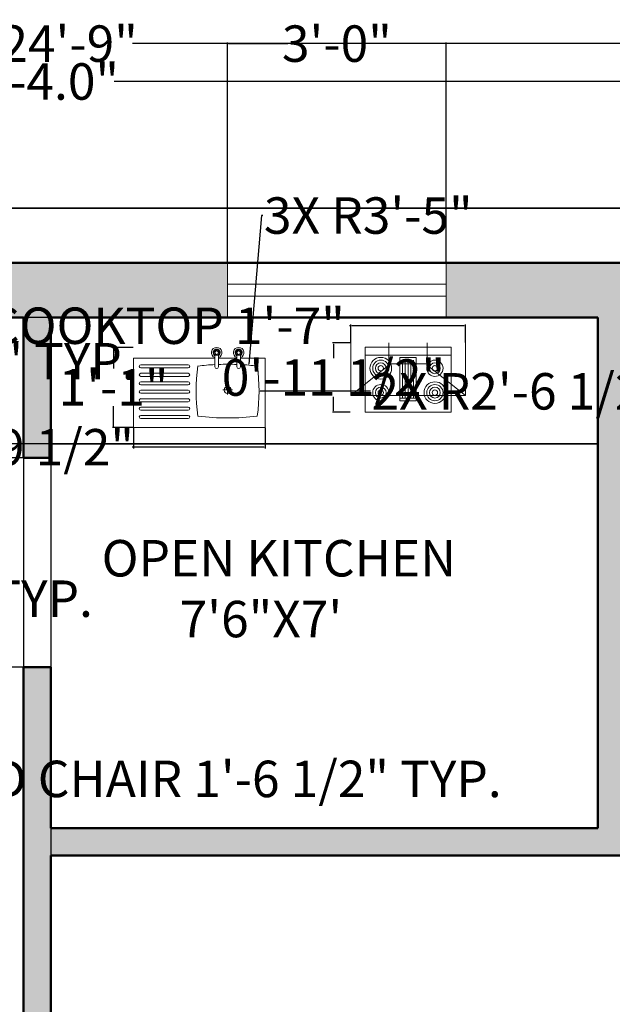
# Model space of a CAD drawing. Units: inches. Extents: x 3398 to 3816, y 15195 to 15771.
# Tile 9 of 10: x 3606 to 3703, y 15609 to 15771. Entities that reach past the tile are written whole.
import ezdxf

# ---------------------------------------------------------------- set-up
doc = ezdxf.new("R2010")
doc.units = ezdxf.units.IN
doc.header["$MEASUREMENT"] = 0
for name, color, linetype, lineweight in [('A-ANNO-DIMS', 2, 'Continuous', 18), ('A-AREA-IDEN', 7, 'Continuous', 25), ('A-EQPM', 8, 'Continuous', 18), ('A-FLOR-CASE', 7, 'Continuous', 25), ('A-FLOR-FIXT', 8, 'Continuous', 18), ('A-GLAZ', 4, 'Continuous', 18), ('A-WALL', 7, 'Continuous', 50), ('A-WALL-PATT', 252, 'Continuous', 13), ('C-PROP', 7, 'Continuous', 35)]:
    doc.layers.add(name, color=color, linetype=linetype, lineweight=lineweight)
doc.styles.get("Standard").update_dxf_attribs({"font": 'arial.ttf'})
doc.dimstyles.get("Standard").update_dxf_attribs({"dimtxt": 6, "dimasz": 0.18, "dimexe": 0.18, "dimexo": 0.0625, "dimgap": 0.09, "dimtad": 0, "dimtih": 1, "dimtoh": 1, "dimdec": 1, "dimzin": 0, "dimdsep": 46, "dimlunit": 3, "dimtxsty": 'Standard', "dimcen": 0.09, "dimadec": 0, "dimazin": 0, "dimtfac": 1, "dimtdec": 1, "dimtofl": 0, "dimtmove": 0, "dimatfit": 3, "dimfxl": 1, "dimtolj": 1, "dimtzin": 0, "dimarcsym": 0})

# ---------------------------------------------------------------- blocks, each defined once
blk = doc.blocks.new('chimmne')
for p, q in [((17.89, 6.07), (-18.11, 6.07)), ((-18.11, 6.07), (-18.11, -10.43)), ((-6.16, -3.43), (-18.11, 6.07)), ((5.94, -3.43), (17.89, 6.07)), ((17.89, 6.07), (17.89, -10.43)), ((-6.16, -3.43), (-6.16, -10.43)), ((5.94, -3.82), (-6.16, -3.82)), ((5.94, -3.43), (5.94, -10.43))]:
    blk.add_line(p, q)
for points in [[(-13.61, -9.12), (-13.61, 11.28), (13.39, 11.28), (13.39, -9.12)], [(-2.66, -5.87), (-2.66, 7.73), (2.44, 7.73), (2.44, -5.87)]]:
    blk.add_lwpolyline(points, close=True)
for points in [[(-2.66, 6.88), (2.44, 6.88)], [(-1.81, 6.88), (-1.81, -5.02)], [(-0.96, -5.02), (-0.96, 6.88)], [(-0.11, 6.88), (-0.11, -5.02)], [(0.74, -5.02), (0.74, 6.88)], [(1.59, 6.88), (1.59, -5.02)], [(13.39, -6.57), (-13.61, -6.57)]]:
    blk.add_lwpolyline(points)
for centre, radius in [((-8.55, 5.18), 3.4), ((-8.55, 5.18), 2.55), ((-8.55, 5.18), 1.7), ((8.44, 5.18), 2.55), ((8.44, 5.18), 1.7), ((-8.55, 5.18), 0.85), ((8.44, 5.18), 0.85), ((-8.55, -2.47), 2.55), ((8.44, -2.47), 3.4), ((8.44, -2.47), 2.55), ((-8.55, -2.47), 1.7), ((-8.55, -2.47), 0.85), ((8.44, -2.47), 1.7), ((8.44, -2.47), 0.85)]:
    blk.add_circle(centre, radius)
blk = doc.blocks.new('A$C799204C7')
for p, q in [((0, 34.2), (17.99, 34.2)), ((0, 0), (0, 34.2)), ((17.99, 13.08), (17.99, 34.2)), ((2.32, 20.01), (2.32, 32.27)), ((3.13, 20.01), (3.13, 32.27)), ((4.48, 20.01), (4.48, 32.27)), ((5.29, 20.01), (5.29, 32.27)), ((6.64, 20.01), (6.64, 32.27)), ((7.45, 20.01), (7.45, 32.27)), ((8.85, 20.01), (8.85, 32.27)), ((9.66, 20.01), (9.66, 32.27)), ((11.01, 20.01), (11.01, 32.27)), ((11.82, 20.01), (11.82, 32.27)), ((13.22, 20.01), (13.22, 32.27)), ((14.03, 20.01), (14.03, 32.27)), ((15.42, 20.01), (15.42, 32.27)), ((16.24, 20.01), (16.24, 32.27)), ((18.59, 13.08), (15.71, 13.08)), ((9.73, 11), (9.73, 8.54)), ((15.71, 12.17), (18.59, 12.17)), ((17.99, 7.36), (17.99, 12.17)), ((8.52, 9.77), (10.9, 9.77)), ((18.59, 7.36), (15.71, 7.36)), ((15.71, 6.45), (18.59, 6.45)), ((17.99, 0), (17.99, 6.45)), ((0, 0), (17.99, 0))]:
    blk.add_line(p, q)
for centre, radius in [((19.38, 12.62), 0.684), ((19.38, 12.62), 0.456), ((9.7, 9.77), 0.916), ((19.38, 6.91), 0.684), ((19.38, 6.91), 0.456)]:
    blk.add_circle(centre, radius)
for centre, radius, start, end in [((2.72, 32.27), 0.407, 0, 180), ((4.88, 32.27), 0.407, 0, 180), ((7.05, 32.27), 0.407, 0, 180), ((9.25, 32.27), 0.407, 0, 180), ((11.42, 32.27), 0.407, 0, 180), ((13.62, 32.27), 0.407, 0, 180), ((15.83, 32.27), 0.407, 0, 180), ((2.72, 20.01), 0.407, 180, 0), ((9.53, -30.19), 48.1, 82.3437, 97.8966), ((4.88, 20.01), 0.407, 180, 0), ((7.05, 20.01), 0.407, 180, 0), ((9.25, 20.01), 0.407, 180, 0), ((11.42, 20.01), 0.407, 180, 0), ((13.62, 20.01), 0.407, 180, 0), ((15.83, 20.01), 0.407, 180, 0), ((67.33, 9.77), 64.88, 173.1952, 186.8048), ((-48.51, 9.77), 64.88, 2.9208, 6.8048), ((15.71, 12.62), 0.456, 90, 270), ((19.38, 12.62), 1.37, 199.6514, 160.3603), ((19.38, 12.62), 0.911, 210.3431, 149.7554), ((-48.51, 9.77), 64.88, 357.8723, 2.115), ((19.38, 6.91), 1.37, 199.6514, 160.3603), ((19.38, 6.91), 0.911, 210.3431, 149.7554), ((15.71, 6.91), 0.456, 90, 270), ((-48.51, 9.77), 64.88, 353.1952, 357.0665), ((9.53, 49.73), 48.1, 262.1034, 277.6563)]:
    blk.add_arc(centre, radius, start, end)
blk = doc.blocks.new('*D4')
at = {"layer": 'A-ANNO-DIMS', "color": 0, "lineweight": -2, "transparency": 16777216}
for p, q in [((3443.19, 15739.58), (3443.19, 15760.52)), ((3771.19, 15739.58), (3771.19, 15760.52)), ((3443.37, 15760.34), (3593.25, 15760.34)), ((3771.01, 15760.34), (3621.13, 15760.34))]:
    blk.add_line(p, q, dxfattribs=at)
at = {"layer": 'A-ANNO-DIMS', "color": 0, "transparency": 16777216}
for points in [[(3443.37, 15760.37), (3443.37, 15760.31), (3443.19, 15760.34)], [(3771.01, 15760.37), (3771.01, 15760.31), (3771.19, 15760.34)]]:
    blk.add_solid(points, dxfattribs=at)
at = {"layer": 'Defpoints', "color": 0, "transparency": 16777216}
for p in [(3771.19, 15760.34), (3443.19, 15739.52), (3771.19, 15739.52)]:
    blk.add_point(p, dxfattribs=at)
at = {"layer": 'A-ANNO-DIMS', "color": 0, "transparency": 16777216, "insert": (3607.19, 15760.34), "char_height": 6, "attachment_point": 5}
blk.add_mtext('\\A1;27\'-4.0"', dxfattribs=at)
blk = doc.blocks.new('*D14')
at = {"layer": 'A-ANNO-DIMS', "color": 0, "lineweight": -2, "transparency": 16777216}
for p, q in [((3515.96, 15721.46), (3515.96, 15714.14)), ((3563.96, 15721.46), (3563.96, 15714.14)), ((3516.14, 15714.32), (3563.78, 15714.32)), ((3563.96, 15714.32), (3564.14, 15714.32))]:
    blk.add_line(p, q, dxfattribs=at)
at = {"layer": 'A-ANNO-DIMS', "color": 0, "transparency": 16777216}
for points in [[(3516.14, 15714.35), (3516.14, 15714.29), (3515.96, 15714.32)], [(3563.78, 15714.35), (3563.78, 15714.29), (3563.96, 15714.32)]]:
    blk.add_solid(points, dxfattribs=at)
at = {"layer": 'Defpoints', "color": 0, "transparency": 16777216}
for p in [(3515.96, 15721.52), (3563.96, 15721.52), (3563.96, 15714.32)]:
    blk.add_point(p, dxfattribs=at)
at = {"layer": 'A-ANNO-DIMS', "color": 0, "transparency": 16777216, "insert": (3595.08, 15714.32), "char_height": 6, "attachment_point": 5}
blk.add_mtext('\\A1;SASH 4\'-0" TYP.', dxfattribs=at)
blk = doc.blocks.new('*D16')
at = {"layer": 'A-ANNO-DIMS', "color": 0, "lineweight": -2, "transparency": 16777216}
for p, q in [((3521.16, 15677.98), (3521.16, 15675.08)), ((3539.72, 15677.98), (3539.72, 15675.08)), ((3521.34, 15675.26), (3539.54, 15675.26)), ((3539.72, 15675.26), (3539.9, 15675.26))]:
    blk.add_line(p, q, dxfattribs=at)
at = {"layer": 'A-ANNO-DIMS', "color": 0, "transparency": 16777216}
for points in [[(3521.34, 15675.29), (3521.34, 15675.23), (3521.16, 15675.26)], [(3539.54, 15675.29), (3539.54, 15675.23), (3539.72, 15675.26)]]:
    blk.add_solid(points, dxfattribs=at)
at = {"layer": 'Defpoints', "color": 0, "transparency": 16777216}
for p in [(3521.16, 15678.04), (3539.72, 15678.04), (3539.72, 15675.26)]:
    blk.add_point(p, dxfattribs=at)
at = {"layer": 'A-ANNO-DIMS', "color": 0, "transparency": 16777216, "insert": (3579.44, 15675.26), "char_height": 6, "attachment_point": 5}
blk.add_mtext('\\A1;CHAIR 1\'-6 1/2" TYP.', dxfattribs=at)
blk = doc.blocks.new('*D18')
at = {"layer": 'A-ANNO-DIMS', "color": 0, "lineweight": -2, "transparency": 16777216}
for p, q in [((3548.56, 15642.88), (3548.56, 15645.79)), ((3548.74, 15645.61), (3566.94, 15645.61)), ((3567.12, 15642.88), (3567.12, 15645.79)), ((3567.12, 15645.61), (3567.3, 15645.61))]:
    blk.add_line(p, q, dxfattribs=at)
at = {"layer": 'A-ANNO-DIMS', "color": 0, "transparency": 16777216}
for points in [[(3548.74, 15645.64), (3548.74, 15645.58), (3548.56, 15645.61)], [(3566.94, 15645.64), (3566.94, 15645.58), (3567.12, 15645.61)]]:
    blk.add_solid(points, dxfattribs=at)
at = {"layer": 'Defpoints', "color": 0, "transparency": 16777216}
for p in [(3567.12, 15645.61), (3548.56, 15642.82), (3567.12, 15642.82)]:
    blk.add_point(p, dxfattribs=at)
at = {"layer": 'A-ANNO-DIMS', "color": 0, "transparency": 16777216, "insert": (3627.67, 15645.61), "char_height": 6, "attachment_point": 5}
blk.add_mtext('\\A1;TRIMMED CHAIR 1\'-6 1/2" TYP.', dxfattribs=at)
blk = doc.blocks.new('*D30')
at = {"layer": 'A-ANNO-DIMS', "color": 0, "lineweight": -2, "transparency": 16777216}
for p, q in [((3660.03, 15720.16), (3659.85, 15720.16)), ((3660.03, 15717.39), (3660.03, 15720.34)), ((3678.72, 15720.16), (3660.21, 15720.16)), ((3678.9, 15717.39), (3678.9, 15720.34))]:
    blk.add_line(p, q, dxfattribs=at)
at = {"layer": 'A-ANNO-DIMS', "color": 0, "transparency": 16777216}
for points in [[(3660.21, 15720.19), (3660.21, 15720.13), (3660.03, 15720.16)], [(3678.72, 15720.19), (3678.72, 15720.13), (3678.9, 15720.16)]]:
    blk.add_solid(points, dxfattribs=at)
at = {"layer": 'Defpoints', "color": 0, "transparency": 16777216}
for p in [(3660.03, 15720.16), (3660.03, 15717.33), (3678.9, 15717.33)]:
    blk.add_point(p, dxfattribs=at)
at = {"layer": 'A-ANNO-DIMS', "color": 0, "transparency": 16777216, "insert": (3629.7, 15720.16), "char_height": 6, "attachment_point": 5}
blk.add_mtext('\\A1;COOKTOP 1\'-7"', dxfattribs=at)
blk = doc.blocks.new('*D31')
at = {"layer": 'A-ANNO-DIMS', "color": 0, "lineweight": -2, "transparency": 16777216}
for p, q in [((3659.97, 15717.33), (3657.02, 15717.33)), ((3657.2, 15717.15), (3657.2, 15714.84)), ((3657.2, 15706.14), (3657.2, 15708.45)), ((3659.97, 15705.96), (3657.02, 15705.96))]:
    blk.add_line(p, q, dxfattribs=at)
at = {"layer": 'A-ANNO-DIMS', "color": 0, "transparency": 16777216}
for points in [[(3657.17, 15717.15), (3657.23, 15717.15), (3657.2, 15717.33)], [(3657.17, 15706.14), (3657.23, 15706.14), (3657.2, 15705.96)]]:
    blk.add_solid(points, dxfattribs=at)
at = {"layer": 'Defpoints', "color": 0, "transparency": 16777216}
for p in [(3660.03, 15717.33), (3657.2, 15705.96), (3660.03, 15705.96)]:
    blk.add_point(p, dxfattribs=at)
at = {"layer": 'A-ANNO-DIMS', "color": 0, "transparency": 16777216, "insert": (3657.2, 15711.64), "char_height": 6, "attachment_point": 5}
blk.add_mtext('\\A1;0\'-11 1/2"', dxfattribs=at)
blk = doc.blocks.new('*D32')
at = {"layer": 'A-ANNO-DIMS', "color": 0, "lineweight": -2, "transparency": 16777216}
for p, q in [((3624.27, 15703.37), (3624.27, 15699.99)), ((3645.98, 15703.37), (3645.98, 15699.99)), ((3624.27, 15700.17), (3624.09, 15700.17)), ((3645.8, 15700.17), (3624.45, 15700.17))]:
    blk.add_line(p, q, dxfattribs=at)
at = {"layer": 'A-ANNO-DIMS', "color": 0, "transparency": 16777216}
for points in [[(3624.45, 15700.2), (3624.45, 15700.14), (3624.27, 15700.17)], [(3645.8, 15700.2), (3645.8, 15700.14), (3645.98, 15700.17)]]:
    blk.add_solid(points, dxfattribs=at)
at = {"layer": 'Defpoints', "color": 0, "transparency": 16777216}
for p in [(3624.27, 15703.43), (3645.98, 15703.43), (3624.27, 15700.17)]:
    blk.add_point(p, dxfattribs=at)
at = {"layer": 'A-ANNO-DIMS', "color": 0, "transparency": 16777216, "insert": (3598.1, 15700.17), "char_height": 6, "attachment_point": 5}
blk.add_mtext('\\A1;SINK 1\'-9 1/2"', dxfattribs=at)
blk = doc.blocks.new('*D33')
at = {"layer": 'A-ANNO-DIMS', "color": 0, "lineweight": -2, "transparency": 16777216}
for p, q in [((3624.21, 15716.6), (3620.83, 15716.6)), ((3621.01, 15716.42), (3621.01, 15713.12)), ((3621.01, 15703.61), (3621.01, 15706.91)), ((3624.21, 15703.43), (3620.83, 15703.43))]:
    blk.add_line(p, q, dxfattribs=at)
at = {"layer": 'A-ANNO-DIMS', "color": 0, "transparency": 16777216}
for points in [[(3620.98, 15716.42), (3621.04, 15716.42), (3621.01, 15716.6)], [(3620.98, 15703.61), (3621.04, 15703.61), (3621.01, 15703.43)]]:
    blk.add_solid(points, dxfattribs=at)
at = {"layer": 'Defpoints', "color": 0, "transparency": 16777216}
for p in [(3621.01, 15716.6), (3624.27, 15716.6), (3624.27, 15703.43)]:
    blk.add_point(p, dxfattribs=at)
at = {"layer": 'A-ANNO-DIMS', "color": 0, "transparency": 16777216, "insert": (3621.01, 15710.02), "char_height": 6, "attachment_point": 5}
blk.add_mtext('\\A1;1\'-1"', dxfattribs=at)
blk = doc.blocks.new('*D36')
at = {"layer": 'A-ANNO-DIMS', "color": 0, "lineweight": -2, "transparency": 16777216}
for p, q in [((3465.19, 15730.58), (3465.19, 15766.75)), ((3465.37, 15766.57), (3603.24, 15766.57)), ((3762.01, 15766.57), (3624.14, 15766.57)), ((3762.19, 15730.58), (3762.19, 15766.75))]:
    blk.add_line(p, q, dxfattribs=at)
at = {"layer": 'A-ANNO-DIMS', "color": 0, "transparency": 16777216}
for points in [[(3465.37, 15766.6), (3465.37, 15766.54), (3465.19, 15766.57)], [(3762.01, 15766.6), (3762.01, 15766.54), (3762.19, 15766.57)]]:
    blk.add_solid(points, dxfattribs=at)
at = {"layer": 'Defpoints', "color": 0, "transparency": 16777216}
for p in [(3762.19, 15766.57), (3465.19, 15730.52), (3762.19, 15730.52)]:
    blk.add_point(p, dxfattribs=at)
at = {"layer": 'A-ANNO-DIMS', "color": 0, "transparency": 16777216, "insert": (3613.69, 15766.57), "char_height": 6, "attachment_point": 5}
blk.add_mtext('\\A1;24\'-9"', dxfattribs=at)
blk = doc.blocks.new('*D42')
at = {"layer": 'A-ANNO-DIMS', "color": 0, "lineweight": -2, "transparency": 16777216}
for p, q in [((3606.19, 15698.39), (3606.19, 15203.29)), ((3610.7, 15698.39), (3610.7, 15203.29)), ((3606.37, 15203.47), (3610.52, 15203.47)), ((3610.7, 15203.47), (3610.88, 15203.47))]:
    blk.add_line(p, q, dxfattribs=at)
at = {"layer": 'A-ANNO-DIMS', "color": 0, "transparency": 16777216}
for points in [[(3606.37, 15203.5), (3606.37, 15203.44), (3606.19, 15203.47)], [(3610.52, 15203.5), (3610.52, 15203.44), (3610.7, 15203.47)]]:
    blk.add_solid(points, dxfattribs=at)
at = {"layer": 'Defpoints', "color": 0, "transparency": 16777216}
for p in [(3606.19, 15698.45), (3610.7, 15698.45), (3610.7, 15203.47)]:
    blk.add_point(p, dxfattribs=at)
at = {"layer": 'A-ANNO-DIMS', "color": 0, "transparency": 16777216, "insert": (3625.93, 15203.47), "char_height": 6, "attachment_point": 5}
blk.add_mtext('\\A1;0\'-4 1/2"', dxfattribs=at)
blk = doc.blocks.new('*D46')
at = {"layer": 'A-ANNO-DIMS', "color": 0, "lineweight": -2, "transparency": 16777216}
for p, q in [((3606.13, 15698.45), (3415.96, 15698.45)), ((3416.14, 15698.27), (3416.14, 15684.4)), ((3416.14, 15664.15), (3416.14, 15678.02)), ((3606.13, 15663.97), (3415.96, 15663.97))]:
    blk.add_line(p, q, dxfattribs=at)
at = {"layer": 'A-ANNO-DIMS', "color": 0, "transparency": 16777216}
for points in [[(3416.11, 15698.27), (3416.17, 15698.27), (3416.14, 15698.45)], [(3416.11, 15664.15), (3416.17, 15664.15), (3416.14, 15663.97)]]:
    blk.add_solid(points, dxfattribs=at)
at = {"layer": 'Defpoints', "color": 0, "transparency": 16777216}
for p in [(3416.14, 15698.45), (3606.19, 15698.45), (3606.19, 15663.97)]:
    blk.add_point(p, dxfattribs=at)
at = {"layer": 'A-ANNO-DIMS', "color": 0, "transparency": 16777216, "insert": (3416.14, 15681.21), "char_height": 6, "attachment_point": 5}
blk.add_mtext('\\A1;2\'-10 1/2"', dxfattribs=at)
blk = doc.blocks.new('*D47')
at = {"layer": 'A-ANNO-DIMS', "color": 0, "lineweight": -2, "transparency": 16777216}
for p, q in [((3639.76, 15730.58), (3639.76, 15766.75)), ((3639.94, 15766.57), (3649.7, 15766.57)), ((3675.58, 15766.57), (3665.83, 15766.57)), ((3675.76, 15730.58), (3675.76, 15766.75))]:
    blk.add_line(p, q, dxfattribs=at)
at = {"layer": 'A-ANNO-DIMS', "color": 0, "transparency": 16777216}
for points in [[(3639.94, 15766.6), (3639.94, 15766.54), (3639.76, 15766.57)], [(3675.58, 15766.6), (3675.58, 15766.54), (3675.76, 15766.57)]]:
    blk.add_solid(points, dxfattribs=at)
at = {"layer": 'Defpoints', "color": 0, "transparency": 16777216}
for p in [(3675.76, 15766.57), (3639.76, 15730.52), (3675.76, 15730.52)]:
    blk.add_point(p, dxfattribs=at)
at = {"layer": 'A-ANNO-DIMS', "color": 0, "transparency": 16777216, "insert": (3657.76, 15766.57), "char_height": 6, "attachment_point": 5}
blk.add_mtext('\\A1;3\'-0"', dxfattribs=at)
blk = doc.blocks.new('*D49')
at = {"layer": 'A-ANNO-DIMS', "color": 0, "lineweight": -2, "transparency": 16777216}
for p, q in [((3700.63, 15721.52), (3415.96, 15721.52)), ((3416.14, 15721.34), (3416.14, 15714.27)), ((3416.14, 15700.89), (3416.14, 15707.96)), ((3700.63, 15700.71), (3415.96, 15700.71))]:
    blk.add_line(p, q, dxfattribs=at)
at = {"layer": 'A-ANNO-DIMS', "color": 0, "transparency": 16777216}
for points in [[(3416.11, 15721.34), (3416.17, 15721.34), (3416.14, 15721.52)], [(3416.11, 15700.89), (3416.17, 15700.89), (3416.14, 15700.71)]]:
    blk.add_solid(points, dxfattribs=at)
at = {"layer": 'Defpoints', "color": 0, "transparency": 16777216}
for p in [(3416.14, 15721.52), (3700.69, 15721.52), (3700.69, 15700.71)]:
    blk.add_point(p, dxfattribs=at)
at = {"layer": 'A-ANNO-DIMS', "color": 0, "transparency": 16777216, "insert": (3416.14, 15711.12), "char_height": 6, "attachment_point": 5}
blk.add_mtext('\\A1;1\'-9"', dxfattribs=at)
blk = doc.blocks.new('*D58')
at = {"layer": 'A-ANNO-DIMS', "color": 0, "lineweight": -2, "transparency": 16777216}
for p, q in [((3645.37, 15738.29), (3643.29, 15713.85)), ((3645.55, 15738.29), (3645.37, 15738.29)), ((3639.69, 15672.63), (3639.87, 15672.63)), ((3639.78, 15672.54), (3639.78, 15672.72))]:
    blk.add_line(p, q, dxfattribs=at)
at = {"layer": 'A-ANNO-DIMS', "color": 0, "transparency": 16777216}
blk.add_solid([(3643.26, 15713.85), (3643.32, 15713.85), (3643.27, 15713.67)], dxfattribs=at)
at = {"layer": 'Defpoints', "color": 0, "transparency": 16777216}
for p in [(3643.27, 15713.67), (3639.78, 15672.63)]:
    blk.add_point(p, dxfattribs=at)
at = {"layer": 'A-ANNO-DIMS', "color": 0, "transparency": 16777216, "insert": (3662.93, 15738.29), "char_height": 6, "attachment_point": 5}
blk.add_mtext('\\A1;3X R3\'-5"', dxfattribs=at)
blk = doc.blocks.new('*D59')
at = {"layer": 'A-ANNO-DIMS', "color": 0, "lineweight": -2, "transparency": 16777216}
for p, q in [((3614.32, 15709.48), (3614.5, 15709.48)), ((3614.41, 15709.39), (3614.41, 15709.57)), ((3663.27, 15709.37), (3645.13, 15709.41))]:
    blk.add_line(p, q, dxfattribs=at)
at = {"layer": 'A-ANNO-DIMS', "color": 0, "transparency": 16777216}
blk.add_solid([(3645.13, 15709.44), (3645.13, 15709.38), (3644.95, 15709.41)], dxfattribs=at)
at = {"layer": 'Defpoints', "color": 0, "transparency": 16777216}
for p in [(3614.41, 15709.48), (3644.95, 15709.41)]:
    blk.add_point(p, dxfattribs=at)
at = {"layer": 'A-ANNO-DIMS', "color": 0, "transparency": 16777216, "insert": (3687.69, 15709.37), "char_height": 6, "attachment_point": 5}
blk.add_mtext('\\A1;2X R2\'-6 1/2"', dxfattribs=at)

msp = doc.modelspace()

# ---------------------------------------------------------------- hatches: boundary and pattern name
at = {"layer": 'A-WALL-PATT'}
h = msp.add_hatch(color=256, dxfattribs=at)
h.dxf.hatch_style = 1
h.paths.add_polyline_path([(3515.96, 15730.52), (3465.19, 15730.52), (3465.19, 15715.52), (3474.19, 15715.52), (3474.19, 15721.52), (3515.96, 15721.52)])
h.paths.add_polyline_path([(3719.81, 15730.52), (3675.76, 15730.52), (3675.76, 15721.52), (3700.69, 15721.52), (3700.69, 15637.52), (3610.69, 15637.52), (3610.69, 15663.97), (3606.19, 15663.97), (3606.19, 15601.52), (3599.08, 15601.52), (3599.08, 15592.52), (3606.19, 15592.52), (3606.19, 15508.52), (3616.69, 15508.52), (3616.69, 15513.02), (3610.69, 15513.02), (3610.69, 15633.02), (3708.19, 15633.02), (3708.19, 15637.52), (3705.19, 15637.52), (3705.19, 15721.52), (3719.81, 15721.52)])
h.paths.add_polyline_path([(3762.19, 15730.52), (3743.77, 15730.52), (3743.77, 15721.52), (3753.19, 15721.52), (3753.19, 15637.52), (3732.19, 15637.52), (3732.19, 15633.02), (3753.19, 15633.02), (3753.19, 15597.39), (3762.19, 15597.39)])
h.paths.add_polyline_path([(3762.19, 15549.39), (3753.19, 15549.39), (3753.19, 15513.02), (3652.69, 15513.02), (3652.69, 15508.52), (3664.69, 15508.52), (3664.69, 15460.52), (3652.69, 15460.52), (3652.69, 15456.02), (3672.19, 15456.02), (3672.19, 15460.52), (3669.19, 15460.52), (3669.19, 15508.52), (3753.19, 15508.52), (3753.19, 15497.51), (3762.19, 15497.51)])
h.paths.add_polyline_path([(3762.19, 15473.48), (3753.19, 15473.48), (3753.19, 15460.52), (3696.19, 15460.52), (3696.19, 15456.02), (3753.19, 15456.02), (3753.19, 15414.25), (3762.19, 15414.25)])
h.paths.add_polyline_path([(3762.19, 15366.28), (3753.19, 15366.28), (3753.19, 15324.02), (3610.69, 15324.02), (3610.69, 15456.02), (3616.69, 15456.02), (3616.69, 15460.52), (3610.69, 15460.52), (3606.19, 15460.52), (3606.19, 15382.52), (3587.73, 15382.52), (3587.73, 15373.52), (3606.19, 15373.52), (3606.19, 15315.02), (3762.19, 15315.02)])
h.paths.add_polyline_path([(3539.73, 15382.52), (3522.19, 15382.52), (3522.19, 15373.52), (3539.73, 15373.52)])
h.paths.add_polyline_path([(3480.19, 15382.52), (3474.19, 15382.52), (3474.19, 15452.47), (3465.19, 15452.47), (3465.19, 15373.52), (3480.19, 15373.52)])
h.paths.add_polyline_path([(3551.04, 15601.52), (3474.19, 15601.52), (3474.19, 15679.52), (3465.19, 15679.52), (3465.19, 15500.47), (3474.19, 15500.47), (3474.19, 15592.52), (3551.04, 15592.52)])
h = msp.add_hatch(color=256, dxfattribs=at)
h.dxf.hatch_style = 1
h.paths.add_polyline_path([(3610.69, 15721.52), (3639.76, 15721.52), (3639.76, 15730.52), (3563.96, 15730.52), (3563.96, 15721.52), (3606.19, 15721.52), (3606.19, 15700.71), (3606.19, 15698.45), (3610.7, 15698.45), (3610.7, 15700.71), (3610.69, 15700.71)])

# ---------------------------------------------------------------- linework, layer by layer
at = {"layer": 'A-FLOR-CASE'}
msp.add_line((3610.69, 15700.71), (3700.69, 15700.71), dxfattribs=at)
at = {"layer": 'A-GLAZ'}
for p, q in [((3639.76, 15730.52), (3639.76, 15721.52)), ((3675.76, 15730.52), (3639.76, 15730.52)), ((3675.76, 15721.52), (3675.76, 15730.52)), ((3675.76, 15727.02), (3639.76, 15727.02)), ((3639.76, 15725.02), (3675.76, 15725.02)), ((3639.76, 15721.52), (3675.76, 15721.52))]:
    msp.add_line(p, q, dxfattribs=at)
at = {"layer": 'A-WALL'}
for p, q in [((3452.19, 15730.52), (3762.19, 15730.52)), ((3474.19, 15721.52), (3606.19, 15721.52)), ((3606.19, 15721.52), (3606.19, 15700.71)), ((3610.69, 15721.52), (3610.69, 15700.71)), ((3610.69, 15721.52), (3700.69, 15721.52)), ((3700.69, 15721.52), (3700.69, 15637.52)), ((3606.19, 15700.71), (3606.19, 15698.45)), ((3610.7, 15698.45), (3610.7, 15700.71)), ((3606.19, 15698.45), (3610.7, 15698.45)), ((3610.69, 15663.97), (3606.19, 15663.97)), ((3606.19, 15663.97), (3606.19, 15601.52)), ((3610.69, 15663.97), (3610.69, 15637.52)), ((3610.69, 15637.52), (3700.69, 15637.52)), ((3610.69, 15633.02), (3753.19, 15633.02)), ((3610.69, 15633.02), (3610.69, 15513.02))]:
    msp.add_line(p, q, dxfattribs=at)
at = {"layer": 'C-PROP'}
msp.add_line((3443.19, 15739.52), (3771.19, 15739.52), dxfattribs=at)

# ---------------------------------------------------------------- block references
at = {"layer": 'A-EQPM', "xscale": 0.5240213531540189, "yscale": 0.5240213531540189, "zscale": 0.5240213531540189, "rotation": 180}
msp.add_blockref('chimmne', (3669.41, 15711.87), dxfattribs=at)
at = {"layer": 'A-FLOR-FIXT', "xscale": 0.6348766007512002, "yscale": 0.6348766007512002, "zscale": 0.6348766007512002, "rotation": 89.99999999999999}
msp.add_blockref('A$C799204C7', (3645.98, 15703.43), dxfattribs=at)

# ---------------------------------------------------------------- texts
at = {"layer": 'A-AREA-IDEN', "insert": (3619.05, 15684.91), "char_height": 6, "attachment_point": 1}
msp.add_mtext_dynamic_manual_height_columns('OPEN KITCHEN\\P       7\'6"X7\'', width=69.833, gutter_width=30, heights=[0], dxfattribs=at)

# ---------------------------------------------------------------- dimensions: what is measured, and where the dimension line sits
at = {"layer": 'A-ANNO-DIMS'}
for base, p1, p2, override, picture, middle in [((3762.19, 15766.57), (3465.19, 15730.52), (3762.19, 15730.52), {"dimdec": 1, "dimlfac": 1, "dimrnd": 0, "dimzin": 1, "dimdsep": 46, "dimlunit": 4, "dimfrac": 2}, '*D36', (3613.69, 15766.57)), ((3675.76, 15766.57), (3639.76, 15730.52), (3675.76, 15730.52), {"dimdec": 1, "dimlfac": 1, "dimrnd": 0, "dimzin": 1, "dimdsep": 46, "dimlunit": 4, "dimfrac": 2}, '*D47', (3657.76, 15766.57)), ((3771.19, 15760.34), (3443.19, 15739.52), (3771.19, 15739.52), {"dimclrd": 0, "dimclre": 0, "dimclrt": 0}, '*D4', (3607.19, 15760.34)), ((3610.7, 15203.47), (3606.19, 15698.45), (3610.7, 15698.45), {"dimdec": 1, "dimlfac": 1, "dimrnd": 0, "dimzin": 1, "dimdsep": 46, "dimlunit": 4, "dimfrac": 2}, '*D42', (3625.93, 15203.47))]:
    dim = msp.add_linear_dim(base=base, p1=p1, p2=p2, dimstyle='Standard', override=override, dxfattribs=at)
    dim.commit()
    dim.dimension.update_dxf_attribs({"geometry": picture, "text_midpoint": middle})
for center, mpoint, text, picture, middle in [((3639.78, 15672.63), (3643.27, 15713.67), '3X <>', '*D58', (3662.93, 15738.29)), ((3614.41, 15709.48), (3644.95, 15709.41), '2X <>', '*D59', (3663.27, 15709.37))]:
    dim = msp.add_radius_dim(center=center, mpoint=mpoint, text=text, dimstyle='Standard', override={"dimdec": 1, "dimlfac": 1, "dimrnd": 0, "dimzin": 1, "dimdsep": 46, "dimlunit": 4, "dimfrac": 2}, dxfattribs=at)
    dim.commit()
    dim.dimension.update_dxf_attribs({"geometry": picture, "text_midpoint": middle, "dimtype": 164})
for base, p1, p2, text, picture, middle in [((3563.96, 15714.32), (3515.96, 15721.52), (3563.96, 15721.52), 'SASH <> TYP.', '*D14', (3595.08, 15714.32)), ((3539.72, 15675.26), (3521.16, 15678.04), (3539.72, 15678.04), 'CHAIR <> TYP.', '*D16', (3579.44, 15675.26)), ((3567.12, 15645.61), (3548.56, 15642.82), (3567.12, 15642.82), 'TRIMMED CHAIR <> TYP.', '*D18', (3627.67, 15645.61))]:
    dim = msp.add_linear_dim(base=base, p1=p1, p2=p2, text=text, dimstyle='Standard', override={"dimdec": 1, "dimlfac": 1, "dimrnd": 0, "dimzin": 1, "dimdsep": 46, "dimlunit": 4, "dimfrac": 2}, dxfattribs=at)
    dim.commit()
    dim.dimension.update_dxf_attribs({"geometry": picture, "text_midpoint": middle})
for base, p1, p2, text, picture, middle in [((3660.03, 15720.16), (3678.9, 15717.33), (3660.03, 15717.33), 'COOKTOP <>', '*D30', (3629.7, 15720.16)), ((3624.27, 15700.17), (3645.98, 15703.43), (3624.27, 15703.43), 'SINK <>', '*D32', (3598.1, 15700.17))]:
    dim = msp.add_linear_dim(base=base, p1=p1, p2=p2, angle=180, text=text, dimstyle='Standard', override={"dimdec": 1, "dimlfac": 1, "dimrnd": 0, "dimzin": 1, "dimdsep": 46, "dimlunit": 4, "dimfrac": 2}, dxfattribs=at)
    dim.commit()
    dim.dimension.update_dxf_attribs({"geometry": picture, "text_midpoint": middle})
for base, p1, p2, angle, picture, middle in [((3416.14, 15721.52), (3700.69, 15700.71), (3700.69, 15721.52), 90, '*D49', (3416.14, 15711.12)), ((3657.2, 15705.96), (3660.03, 15717.33), (3660.03, 15705.96), 270, '*D31', (3657.2, 15711.64)), ((3621.01, 15716.6), (3624.27, 15703.43), (3624.27, 15716.6), 90, '*D33', (3621.01, 15710.02)), ((3416.14, 15698.45), (3606.19, 15663.97), (3606.19, 15698.45), 90, '*D46', (3416.14, 15681.21))]:
    dim = msp.add_linear_dim(base=base, p1=p1, p2=p2, angle=angle, dimstyle='Standard', override={"dimdec": 1, "dimlfac": 1, "dimrnd": 0, "dimzin": 1, "dimdsep": 46, "dimlunit": 4, "dimfrac": 2}, dxfattribs=at)
    dim.commit()
    dim.dimension.update_dxf_attribs({"geometry": picture, "text_midpoint": middle})

doc.saveas('drawing.dxf')
